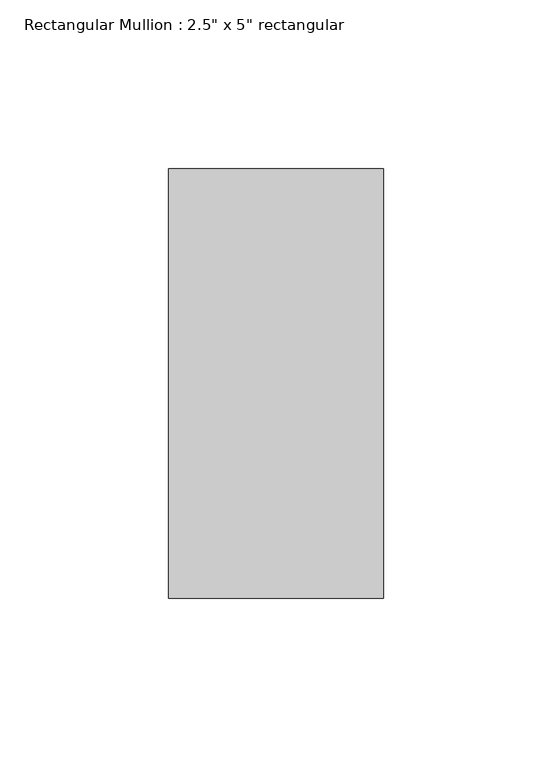
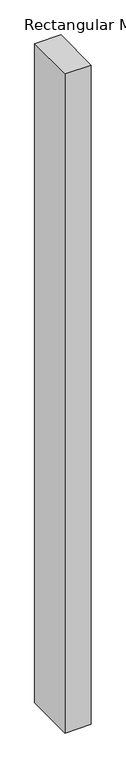
"""IFC4 building model written with IfcOpenShell, lengths in millimetres: member geometry."""

from ifc_helpers import new_model, si_unit, frame, origin, place, context, project, spatial, polyline, outline, extrude, source, transform, mapped, element, save


def member_e74a93ea(model_context):
    return source(origin(), model_context, "Body", "SweptSolid", [
        extrude(outline(polyline([(0.0, 63.5), (0.0, -63.5), (-63.5, -63.5), (-63.5, 63.5), (0.0, 63.5)])), frame((0.0, 0.0, -1686.8910355), z_axis=(0.0, 0.0, 1.0), x_axis=(1.0, 0.0, 0.0)), (0.0, 0.0, 1.0), 1686.8910355),
    ])


if __name__ == "__main__":
    model = new_model("IFC4")
    model_context = context("Model", 3, world=origin())
    ifc_project = project(units=[si_unit("LENGTHUNIT", "METRE", prefix="MILLI")], contexts=[model_context])
    site = spatial("IfcSite", under=ifc_project)
    building = spatial("IfcBuilding", under=site)
    placement = place(None, origin())
    member_shape = member_e74a93ea(model_context)
    element("IfcMember", 1, ObjectType="Rectangular Mullion : 2.5\" x 5\" rectangular", at=placement, inside=building, context=model_context, shape_type="MappedRepresentation", body=[
        mapped(member_shape, transform((0.0, 0.0, 0.0), x_axis=(1.0, 0.0, 0.0), y_axis=(0.0, 1.0, 0.0), z_axis=(0.0, 0.0, 1.0))),
    ])
    save(model, "model.ifc")

# Revit data of these elements
# Type "Rectangular Mullion : 2.5\" x 5\" rectangular"
#   built-in parameter 1007304 = 0.416667 (stored number, unit not read)
#   built-in parameter 1007301 = 0.104167 (stored number, unit not read)
#   built-in parameter 1007300 = 0.104167 (stored number, unit not read)
# Element 1 (IfcMember, "Rectangular Mullion : 2.5\" x 5\" rectangular")
#   Materials on its faces: "Aluminum"
# Materials
#   "Aluminum": class "Metal", colour RGB 247 247 247, transparency 0, Description = "Aluminum 6061", Cost = 0
